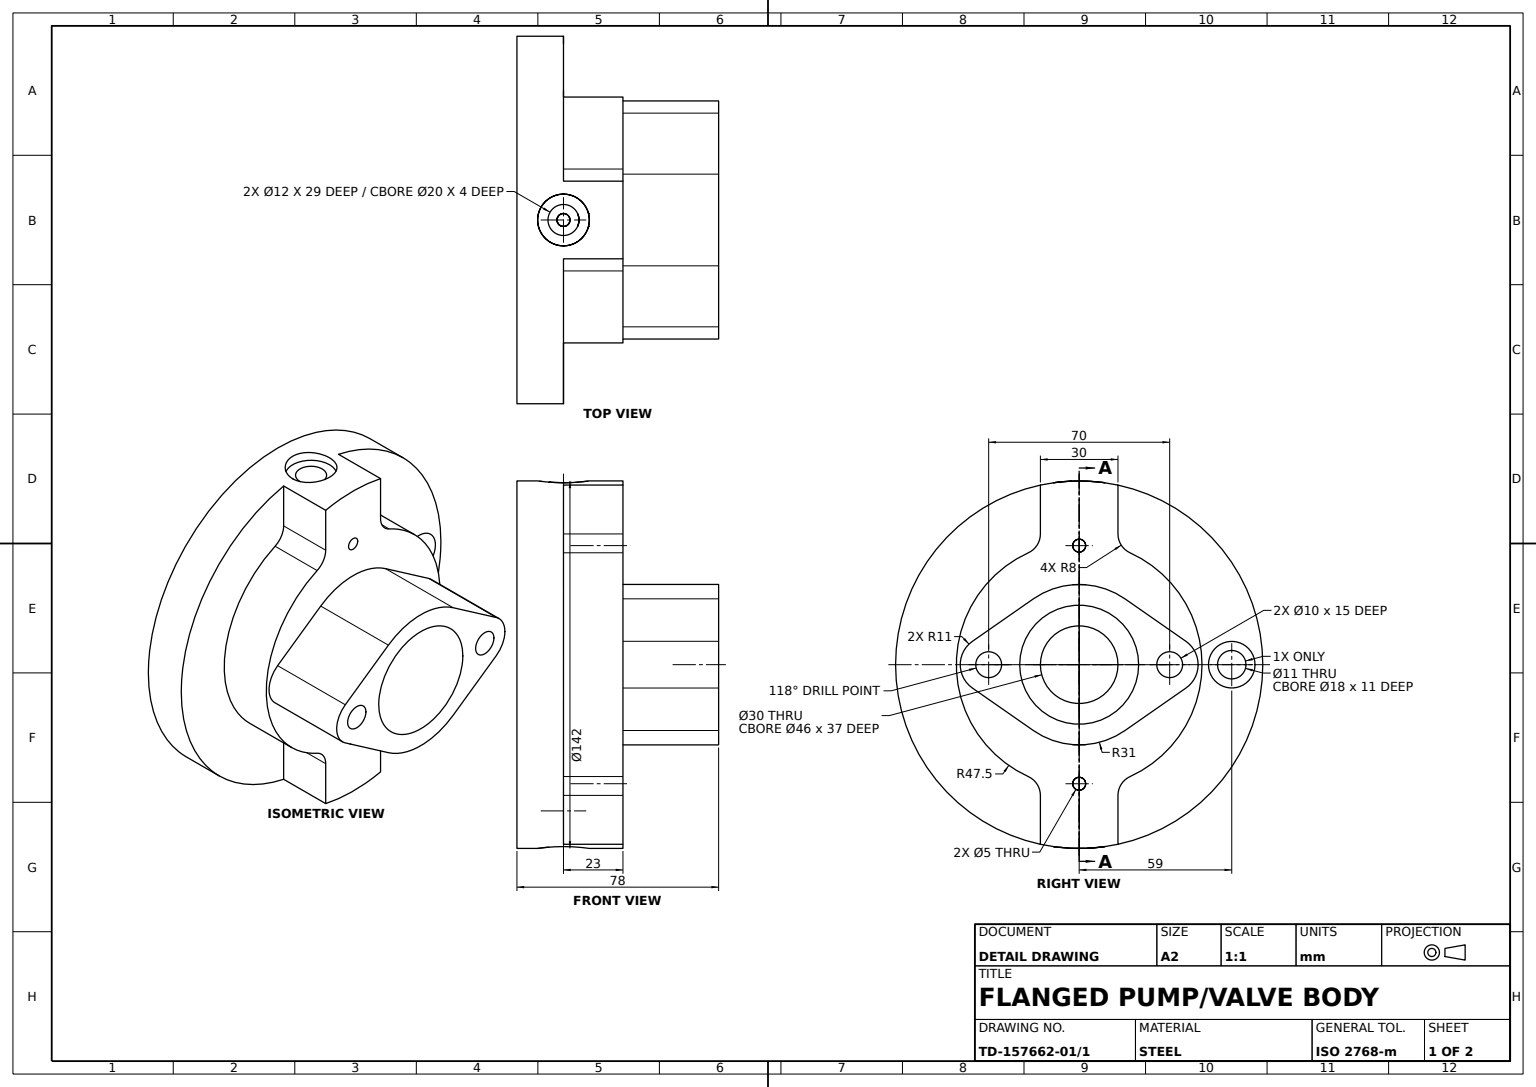
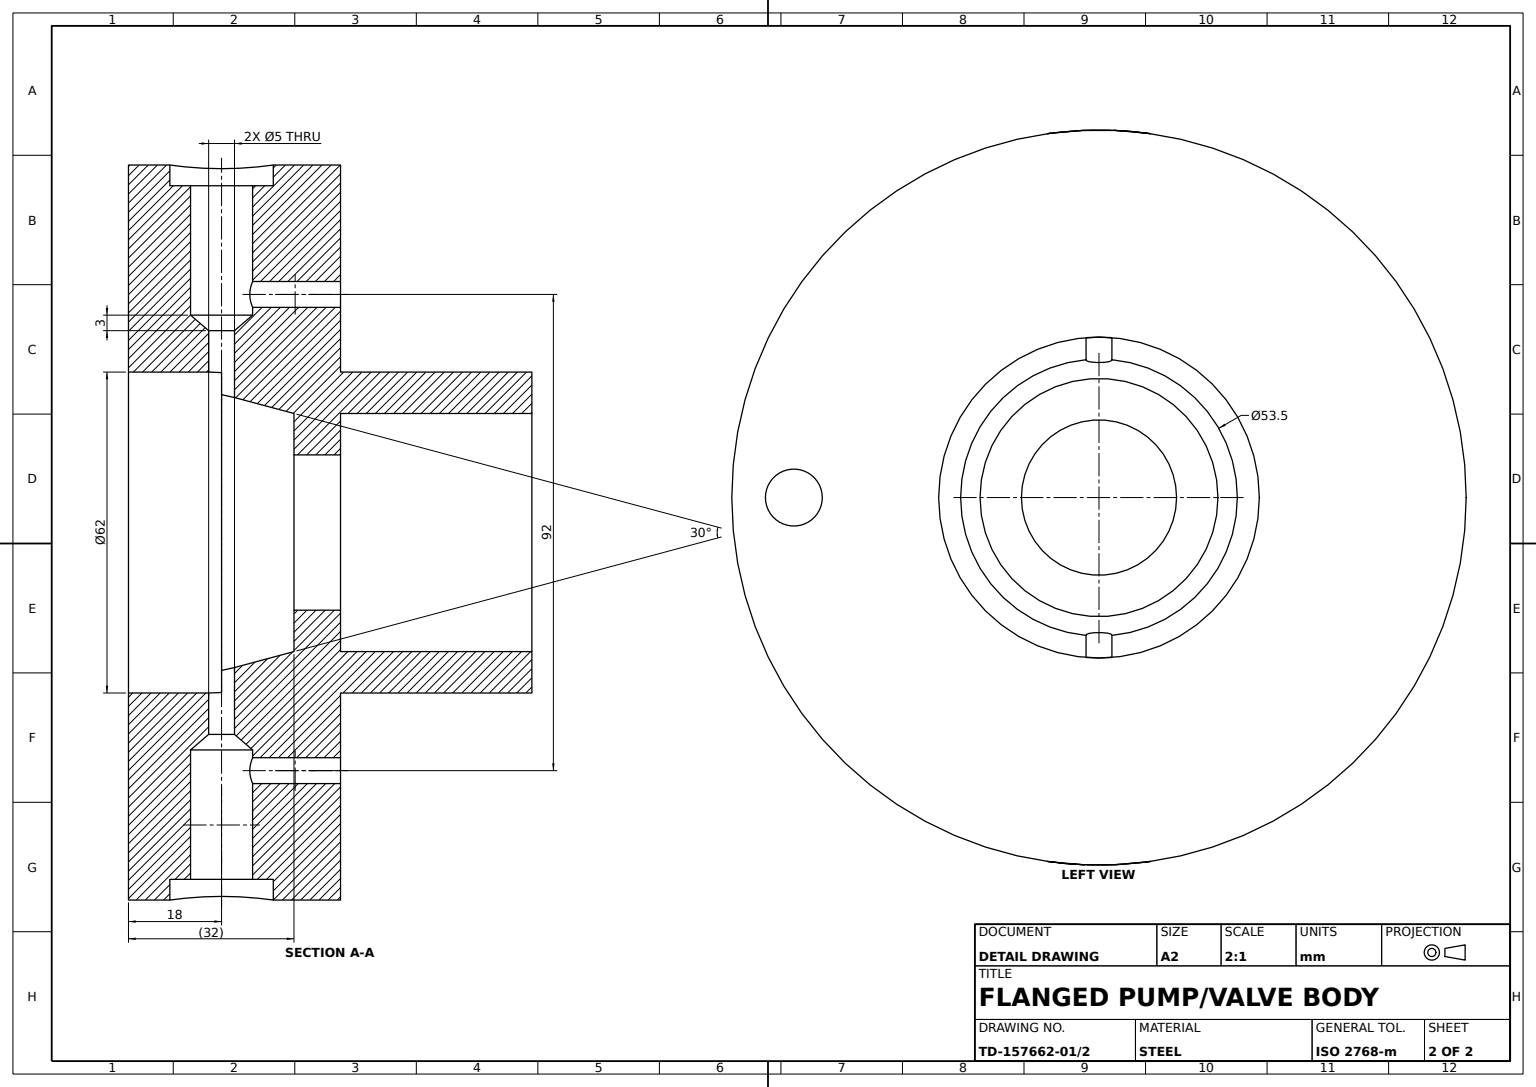
from build123d import *

# Parameters (mm, degrees)
HOUSING_PROFILE_SKETCH_R              = 71
MOUNTING_FLANGE_142_DEPTH             = 18
BODY_START                            = 18
BODY_BOSS_WITH_SIDE_LUGS_DEPTH        = 23
UPPER_START                           = 41
SKETCH1_5_R                           = 23
UPPER_BEARING_BOSS_DEPTH              = 37
BOSS_FILLET_R8_R                      = 8
FLANGE_HOLES_6X_11_C_BORE_D           = 11
FLANGE_HOLES_6X_11_C_BORE_CBORE_D     = 18
FLANGE_HOLES_6X_11_C_BORE_CBORE_DEPTH = 11
SIDE_PORT_12_C_BORE_D                 = 12
SIDE_PORT_12_C_BORE_DEPTH             = 29
SIDE_PORT_12_C_BORE_CBORE_D           = 20
SIDE_PORT_12_C_BORE_CBORE_DEPTH       = 4
SIDE_PORT_RELIEF_CUT_DEPTH            = 128.145585958
SIDE_PORT_RELIEF_CUT_DEPTH_BACK       = 128.145585958
SIDE_PORT_RELIEF_SKETCH_R             = 2.5
UPPER_BOSS_HOLES_10_D                 = 10
UPPER_BOSS_HOLES_10_DEPTH             = 15
UPPER_BOSS_HOLES_10_TIP               = 3.004303095
LUBE_HOLE_5_REACH                     = 110.457
LUBE_HOLE_5_BORE_R                    = 2.5


with BuildPart() as part:
    # Housing Profile Sketch → Mounting Flange _142 (new body)
    with BuildSketch(Plane(origin=(0, 0, 0), x_dir=(1, 0, 0), z_dir=(0, 1, 0))):
        with Locations(Location((0, 0, 0), (0, 0, 270))):
            Circle(HOUSING_PROFILE_SKETCH_R)
    extrude(amount=MOUNTING_FLANGE_142_DEPTH)

    # Sketch1_3 → Body Boss with Side Lugs (add)
    with BuildSketch(Plane(origin=(0, 0, 0), x_dir=(1, 0, 0), z_dir=(0, 1, 0)).offset(BODY_START)):
        with BuildLine():
            ThreePointArc((45.069390943, 15), (0, 47.5), (-45.069390943, 15))
            Line((-45.069390943, 15), (-69.397406292, 15))
            ThreePointArc((-69.397406292, 15), (-71, 0), (-69.397406292, -15))
            Line((-69.397406292, -15), (-45.069390943, -15))
            ThreePointArc((-45.069390943, -15), (0, -47.5), (45.069390943, -15))
            Line((45.069390943, -15), (69.397406292, -15))
            ThreePointArc((69.397406292, -15), (71, 0), (69.397406292, 15))
            Line((69.397406292, 15), (45.069390943, 15))
        make_face()
    extrude(amount=BODY_BOSS_WITH_SIDE_LUGS_DEPTH)

    # Sketch1_5 → Upper Bearing Boss (add)
    with BuildSketch(Plane(origin=(0, 0, 0), x_dir=(1, 0, 0), z_dir=(0, 1, 0)).offset(UPPER_START)):
        with BuildLine():
            Line((25.440206006, -17.714285714), (9.027169873, -41.285714286))
            ThreePointArc((9.027169873, -41.285714286), (0, -46), (-9.027169873, -41.285714286))
            Line((-9.027169873, -41.285714286), (-25.440206006, -17.714285714))
            ThreePointArc((-25.440206006, -17.714285714), (-31, 0), (-25.440206006, 17.714285714))
            Line((-25.440206006, 17.714285714), (-9.027169873, 41.285714286))
            ThreePointArc((-9.027169873, 41.285714286), (0, 46), (9.027169873, 41.285714286))
            Line((9.027169873, 41.285714286), (25.440206006, 17.714285714))
            ThreePointArc((25.440206006, 17.714285714), (31, 0), (25.440206006, -17.714285714))
        make_face()
        with Locations(Location((0, 0, 0), (0, 0, 270))):
            Circle(SKETCH1_5_R, mode=Mode.SUBTRACT)
    extrude(amount=UPPER_BEARING_BOSS_DEPTH)

    # Boss Fillet R8
    boss_fillet_r8_edges = [part.edges().sort_by_distance(p)[0] for p in [
        (45.069390943, 29.5, -15),
        (-45.069390943, 29.5, -15),
        (-45.069390943, 29.5, 15),
        (45.069390943, 29.5, 15),
    ]]
    fillet(boss_fillet_r8_edges, radius=BOSS_FILLET_R8_R)

    # Flange Holes 6x_11 C-Bore (through all)
    with Locations(Plane(origin=(0, 18, 0), x_dir=(1, 0, 0), z_dir=(0, 1, 0))):
        with Locations((0, 59)):
            CounterBoreHole(FLANGE_HOLES_6X_11_C_BORE_D / 2, FLANGE_HOLES_6X_11_C_BORE_CBORE_D / 2, FLANGE_HOLES_6X_11_C_BORE_CBORE_DEPTH)

    # Bearing Bore Profile → Bearing Bore (revolve, cut)
    with BuildSketch(Plane.XY, mode=Mode.PRIVATE) as bearing_bore_sk:
        Polygon((-31, 0), (-31, 18), (-26.751288694, 18), (-23, 32), (-15, 32), (-15, 41), (0, 41), (0, 0), align=None)
    revolve(bearing_bore_sk.sketch.rotate(Axis((0, 0, 0), (0, 1, 0)), 270), axis=Axis((0, 0, 0), (0, 1, 0)), mode=Mode.SUBTRACT)

    # Side Port _12 C-Bore
    with Locations(Plane(origin=(71, 18, 0), x_dir=(0, 0, 1), z_dir=(1, 0, 0))):
        with Locations((0, 0)):
            side_port_12_c_bore = CounterBoreHole(SIDE_PORT_12_C_BORE_D / 2, SIDE_PORT_12_C_BORE_CBORE_D / 2, SIDE_PORT_12_C_BORE_CBORE_DEPTH, depth=SIDE_PORT_12_C_BORE_DEPTH)

    # Side Port Relief Sketch → Side Port Relief Cut (cut, two sides: drawn at the far end of the back side and taken through both)
    with BuildSketch(Plane(origin=(0, 0, 0), x_dir=(0, 0, -1), z_dir=(1, 0, 0)).offset(-SIDE_PORT_RELIEF_CUT_DEPTH_BACK)):
        with Locations(Location((0, 18, 0), (0, 0, 180))):
            Circle(SIDE_PORT_RELIEF_SKETCH_R)
    extrude(amount=SIDE_PORT_RELIEF_CUT_DEPTH + SIDE_PORT_RELIEF_CUT_DEPTH_BACK, mode=Mode.SUBTRACT)

    # Side Port Groove Profile → Side Port Groove (revolve, cut)
    with BuildSketch(Plane.XY, mode=Mode.PRIVATE) as side_port_groove_sk:
        Polygon((42, 12), (39, 15.5), (39, 18), (42, 18), align=None)
    side_port_groove = revolve(side_port_groove_sk.sketch.rotate(Axis((39, 18, 0), (1, 0, 0)), 90), axis=Axis((39, 18, 0), (1, 0, 0)), mode=Mode.SUBTRACT)

    # Side Port Mirror: Side Port _12 C-Bore, Side Port Groove across plane
    add(side_port_12_c_bore.mirror(Plane(origin=(0, 0, 0), x_dir=(0, 0, 1), z_dir=(1, 0, 0))), mode=Mode.SUBTRACT)
    add(side_port_groove.mirror(Plane(origin=(0, 0, 0), x_dir=(0, 0, 1), z_dir=(1, 0, 0))), mode=Mode.SUBTRACT)

    # Upper Boss Holes _10
    with Locations(Plane(origin=(0, 78, 0), x_dir=(1, 0, 0), z_dir=(0, 1, 0))):
        with Locations((0, 35), (0, -35)):
            Hole(UPPER_BOSS_HOLES_10_D / 2, depth=UPPER_BOSS_HOLES_10_DEPTH)
            with Locations((0, 0, -(UPPER_BOSS_HOLES_10_DEPTH + UPPER_BOSS_HOLES_10_TIP / 2))):  # 118° drill point
                Cone(0, UPPER_BOSS_HOLES_10_D / 2, UPPER_BOSS_HOLES_10_TIP, mode=Mode.SUBTRACT)

    # Lube Hole _5 bore → Lube Hole _5 (cut, up to next)
    with BuildSketch(Plane(origin=(0, 41, 0), x_dir=(1, 0, 0), z_dir=(0, 1, 0)), mode=Mode.PRIVATE) as lube_hole_5_sk1:
        with Locations((46, 0)):
            Circle(LUBE_HOLE_5_BORE_R)
    lube_hole_5_tool1 = extrude(lube_hole_5_sk1.sketch, amount=-LUBE_HOLE_5_REACH, mode=Mode.PRIVATE) & part.part
    # Lube Hole _5 bore → Lube Hole _5 (cut, up to next)
    with BuildSketch(Plane(origin=(0, 41, 0), x_dir=(1, 0, 0), z_dir=(0, 1, 0)), mode=Mode.PRIVATE) as lube_hole_5_sk2:
        with Locations((-46, 0)):
            Circle(LUBE_HOLE_5_BORE_R)
    lube_hole_5_tool2 = extrude(lube_hole_5_sk2.sketch, amount=-LUBE_HOLE_5_REACH, mode=Mode.PRIVATE) & part.part
    add(lube_hole_5_tool1.solids().sort_by_distance((46, 41, 0))[0], mode=Mode.SUBTRACT)
    add(lube_hole_5_tool2.solids().sort_by_distance((-46, 41, 0))[0], mode=Mode.SUBTRACT)


solid = part.part
